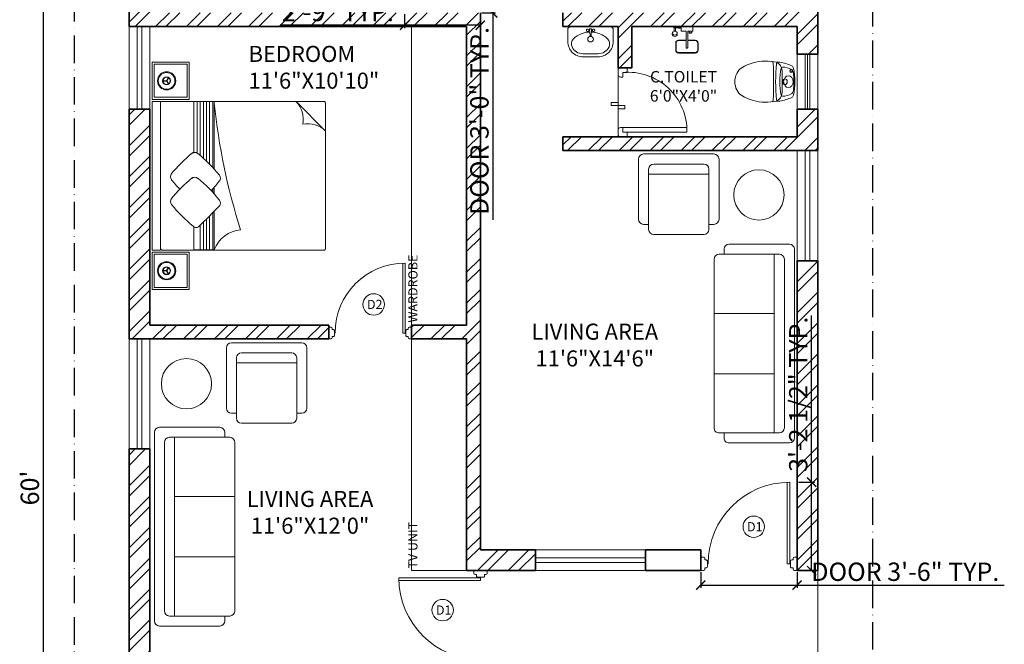
# Model space of a CAD drawing. Units: inches. Extents: x -15 to 1053, y -1 to 793.
# Tile 2 of 8: x 21 to 450, y 337 to 609. Entities that reach past the tile are written whole.
import ezdxf

# ---------------------------------------------------------------- set-up
doc = ezdxf.new("R2010")
doc.units = ezdxf.units.IN
doc.linetypes.add('ACAD_ISO10W100', pattern=[18, 12, -3, 0, -3])
for name, color, linetype, lineweight in [('00 FURNITURE', 15, 'Continuous', 15), ('A-ANNO-DIMS', 2, 'Continuous', 18), ('A-ANNO-TEXT', 7, 'Continuous', 18), ('A-AREA-IDEN', 7, 'Continuous', 18), ('A-DOOR', 4, 'Continuous', 18), ('A-FLOR-CASE', 5, 'Continuous', 18), ('A-FLOR-FIXT', 8, 'Continuous', 13), ('A-FLOR-STRS', 3, 'Continuous', 18), ('A-FURN', 8, 'Continuous', 13), ('A-GLAZ', 4, 'Continuous', 18), ('A-WALL', 7, 'Continuous', 35), ('A-WALL-PATT', 8, 'Continuous', 13), ('A_FUR 1', 5, 'Continuous', 5), ('C-PROP', 1, 'ACAD_ISO10W100', 25)]:
    doc.layers.add(name, color=color, linetype=linetype, lineweight=lineweight)
doc.styles.add('1-100DIM', font='txt', dxfattribs={"height": 0.3})
doc.styles.get("Standard").update_dxf_attribs({"font": 'arial.ttf'})
doc.dimstyles.new('ISO-25', dxfattribs={"dimtxt": 8, "dimasz": 4, "dimexe": 1.25, "dimexo": 0.625, "dimtad": 1, "dimdec": 0, "dimlunit": 4, "dimtxsty": 'Standard', "dimblk": 'ARCHTICK', "dimcen": 3, "dimadec": 0, "dimazin": 0, "dimtfac": 1, "dimtdec": 0, "dimtmove": 0, "dimatfit": 3, "dimldrblk": 'ARCHTICK', "dimfxl": 1, "dimarcsym": 0})

# ---------------------------------------------------------------- blocks, each defined once
blk = doc.blocks.new('s_14')
at = {"extrusion": (0, 0, -1)}
for centre, major_axis, start_param, end_param in [((0, -522), (652, 0), 4.476887, 4.947891), ((0, -522), (652, 0), 4.476887, 4.947891), ((681, -279), (914, 0), 3.289642, 3.481728), ((681, -279), (914, 0), 3.289642, 3.481728), ((-143, -45), (39.1, 0), 3.481728, 4.476887), ((-143, -45), (39.1, 0), 3.481728, 4.476887), ((118, -139), (285, 0), 3.130806, 3.616946), ((-125, -42), (19.2, 0), 3.141593, 9.424778), ((-125, -42), (12.2, 0), 3.141593, 9.424778), ((-97, -51), (42.5, 0), 3.616946, 4.577347), ((0, -624), (766, 0), 4.577347, 4.847431), ((0, -74), (67.1, 0), 3.141593, 9.424778), ((0, -113), (32.9, 0), 3.141593, 9.424778), ((97, -51), (42.5, 0), -1.435755, -0.475353), ((-118, -139), (285, 0), -0.475353, 0.010787), ((143, -45), (39.1, 0), -1.335294, -0.340135), ((143, -45), (39.1, 0), -1.335294, -0.340135), ((-682, -278), (914, 0), -0.340135, -0.148049), ((-682, -278), (914, 0), -0.340135, -0.148049), ((999, -342), (1233, -1), 3.141593, 3.282422), ((999, -342), (1233, -1), 3.141593, 3.282422), ((-87, -187), (137, 0), 3.032389, 3.289642), ((-87, -187), (137, 0), 3.032389, 3.289642), ((-207, -197), (16, 0), 1.680926, 3.032389), ((-207, -197), (16, 0), 1.680926, 3.032389), ((-121, -225), (98.7, 0), 3.365215, 4.657014), ((1, 1302), (1900, -1), 1.460666, 1.680926), ((1, 1302), (1900, -1), 1.460666, 1.680926), ((-149, -142), (17.9, 0), 1.839297, 3.130806), ((0, 291), (579, 0), 1.302296, 1.839297), ((-1, -1970), (2282, -1), 4.657014, 4.767764), ((121, -225), (98.7, 0), -1.515421, -0.223622), ((149, -142), (17.9, 0), 0.010787, 1.302296), ((207, -197), (16, 0), 0.109204, 1.460666), ((207, -197), (16, 0), 0.109204, 1.460666), ((-1000, -341), (1233, -1), -0.140829, 0), ((-1000, -341), (1233, -1), -0.140829, 0), ((87, -187), (137, 0), -0.148049, 0.109204), ((87, -187), (137, 0), -0.148049, 0.109204), ((-210, -263), (19.7, 0), 3.222651, 4.658459), ((-2, -3376), (3914, -2), 4.658459, 4.766319), ((210, -263), (19.7, 0), -1.516867, -0.081058), ((527, -342), (761, 0), 2.693443, 3.141593), ((527, -342), (761, 0), 2.693443, 3.141593), ((-527, -341), (761, 0), 0, 0.44815), ((-527, -341), (761, 0), 0, 0.44815), ((0, -544), (176, 0), 0.44815, 2.693443), ((0, -544), (176, 0), 0.44815, 2.693443)]:
    blk.add_ellipse(centre, major_axis=major_axis, ratio=0.800511, start_param=start_param, end_param=end_param, dxfattribs=at)
blk = doc.blocks.new('s_46')
at = {"ltscale": 600}
h = blk.add_hatch(color=256, dxfattribs=at)
edge = h.paths.add_edge_path()
edge.add_line((13.5, 62), (14.2, 54.1))
edge.add_ellipse((4.2, 52.3), major_axis=(-10.1, 0), ratio=1, start_angle=540, end_angle=550.17546, ccw=False)
edge.add_arc((4.2, 52.3), 10.1, 270, 360, ccw=False)
edge.add_line((4.2, 42.2), (4.2, 41.3))
edge.add_line((4.2, 41.3), (11.9, 41.3))
edge.add_arc((4.2, 52.3), 13.4, 664.69813, 766.48477)
h.paths.add_polyline_path([(4.2, 41.3), (-3.4, 41.3, 0.152567), (4.2, 38.9)])
h.paths.add_polyline_path([(11.9, 41.3), (4.2, 41.3), (4.2, 38.9, 0.152567)])
h.paths.add_polyline_path([(-5.7, 54.1), (-5, 62, 0.475833), (-3.4, 41.3), (4.2, 41.3), (4.2, 42.2, -0.46724)])
for p, q in [((-5.9, 52.3), (-0.7, 110.5)), ((-5.9, 52.3), (-0.7, 110.5)), ((9.1, 110.5), (14.2, 54.1)), ((14.3, 52.3), (9.1, 110.5)), ((14.2, 54.1), (14.3, 52.3))]:
    blk.add_line(p, q, dxfattribs=at)
blk.add_lwpolyline([(-220.8, 171.3, -0.414214), (-70.8, 321.3), (79.2, 321.3, -0.414214), (229.2, 171.3), (229.2, 41.3), (209.2, 21.3), (-200.8, 21.3), (-220.8, 41.3)], format="xyb", close=True, dxfattribs=at)
blk.add_lwpolyline([(12.3, 75.4, 0.181638), (172.2, 141.5, 0.326351), (187.7, 222.7, 0.289814), (79.2, 291.3), (-70.8, 291.3, 0.289814), (-179.2, 222.7, 0.326351), (-163.8, 141.5, 0.181638), (-3.8, 75.4)], format="xyb", dxfattribs=at)
for points in [[(-16.8, 67.4), (-17, 67.5), (-17.2, 67.6), (-17.4, 67.6), (-17.6, 67.7), (-17.8, 67.8), (-18, 67.9), (-18.1, 68.1), (-18.2, 68.2), (-18.3, 68.4), (-18.4, 68.6), (-18.5, 68.8), (-18.7, 68.9), (-18.8, 69.1), (-18.9, 69.2), (-19.1, 69.3), (-19.3, 69.3), (-19.5, 69.3), (-19.7, 69.4), (-19.9, 69.4), (-20.1, 69.4), (-20.3, 69.4), (-20.5, 69.5), (-20.7, 69.6), (-20.8, 69.7), (-21, 69.9), (-21.1, 70), (-21.3, 70.2), (-21.4, 70.3), (-21.5, 70.4), (-21.7, 70.5), (-21.9, 70.5), (-22.1, 70.5), (-22.3, 70.5), (-22.5, 70.5), (-22.7, 70.4), (-22.9, 70.4), (-23.1, 70.4), (-23.3, 70.4), (-23.5, 70.5), (-23.7, 70.6), (-23.9, 70.7), (-24, 70.8), (-24.2, 70.9), (-24.4, 71), (-24.6, 71.1), (-24.7, 71.1), (-24.9, 71.1), (-25.1, 71), (-25.3, 71), (-25.5, 70.9), (-25.7, 70.8), (-25.9, 70.7), (-26.1, 70.6), (-26.3, 70.6), (-26.5, 70.6), (-26.7, 70.6), (-26.9, 70.7), (-27.1, 70.8), (-27.3, 70.8), (-27.5, 70.9), (-27.7, 70.9), (-27.8, 70.9), (-28, 70.8), (-28.2, 70.8), (-28.3, 70.6), (-28.5, 70.5), (-28.7, 70.4), (-28.9, 70.3), (-29.1, 70.2), (-29.3, 70.1), (-29.6, 70.1), (-29.9, 70.1), (-30.2, 70.1), (-30.5, 70), (-30.8, 69.8), (-31.1, 69.5), (-31.4, 69), (-31.6, 68.4), (-32.3, 68.5), (-32.8, 68.4), (-33.2, 68.3), (-33.5, 68.1), (-33.7, 67.8), (-33.9, 67.6), (-34, 67.3), (-34.1, 67.1), (-34.3, 66.9), (-34.5, 66.7), (-34.7, 66.6), (-34.9, 66.5), (-35.1, 66.4), (-35.2, 66.3), (-35.4, 66.2), (-35.5, 66), (-35.6, 65.9), (-35.6, 65.7), (-35.7, 65.5), (-35.7, 65.3), (-35.7, 65.1), (-35.8, 64.9), (-35.8, 64.7), (-35.9, 64.5), (-36, 64.3), (-36.2, 64.2), (-36.3, 64), (-36.5, 63.9), (-36.6, 63.8), (-36.8, 63.6), (-36.9, 63.5), (-37, 63.3), (-37, 63.1), (-37, 63), (-37, 62.8), (-37, 62.6), (-37, 62.3), (-37, 62.1), (-37, 61.9), (-37, 61.7), (-37.1, 61.5), (-37.2, 61.4), (-37.3, 61.2), (-37.4, 61), (-37.5, 60.8), (-37.6, 60.7), (-37.7, 60.5), (-37.8, 60.3), (-37.8, 60.1), (-37.7, 60), (-37.7, 59.8), (-37.6, 59.6), (-37.5, 59.4), (-37.4, 59.2), (-37.4, 59), (-37.4, 58.8), (-37.4, 58.6), (-37.4, 58.4), (-37.5, 58.2), (-37.6, 58), (-37.7, 57.8), (-37.7, 57.6), (-37.8, 57.4), (-37.8, 57.2), (-37.7, 57.1), (-37.6, 56.9), (-37.5, 56.7), (-37.4, 56.6), (-37.3, 56.4), (-37.2, 56.2), (-37.1, 56), (-37, 55.8), (-37, 55.6), (-37, 55.4), (-37, 55.2), (-37, 55), (-37, 54.8), (-37, 54.6), (-37, 54.4), (-37, 54.2), (-36.9, 54.1), (-36.8, 53.9), (-36.6, 53.8), (-36.5, 53.7), (-36.3, 53.5), (-36.2, 53.4), (-36, 53.2), (-35.9, 53.1), (-35.8, 52.9), (-35.8, 52.7), (-35.7, 52.5), (-35.7, 52.3), (-35.7, 52.1), (-35.6, 51.9), (-35.6, 51.7), (-35.5, 51.5), (-35.4, 51.4), (-35.2, 51.3), (-35.1, 51.2), (-34.9, 51.1), (-34.7, 51), (-34.5, 50.9), (-34.3, 50.8), (-34.2, 50.7), (-34, 50.5), (-33.9, 50.3), (-33.8, 50.1), (-33.8, 49.9), (-33.7, 49.8), (-33.6, 49.6), (-33.5, 49.4), (-33.4, 49.3), (-33.2, 49.2), (-33.1, 49.1), (-32.9, 49.1), (-32.7, 49), (-32.5, 49), (-32.2, 48.9), (-32.1, 48.9), (-31.9, 48.8), (-31.7, 48.7), (-31.6, 48.5), (-31.4, 48.3), (-31.3, 48.2), (-31.2, 48), (-31.1, 47.9), (-30.9, 47.7), (-30.8, 47.6), (-30.6, 47.6), (-30.4, 47.5), (-30.2, 47.5), (-30, 47.6), (-29.8, 47.6), (-29.6, 47.6), (-29.4, 47.6), (-29.2, 47.5), (-29, 47.4), (-28.8, 47.3), (-28.7, 47.2), (-28.5, 47.1), (-28.3, 46.9), (-28.2, 46.8), (-28, 46.7), (-27.8, 46.7), (-27.7, 46.7), (-27.5, 46.7), (-27.3, 46.7), (-27.1, 46.8), (-26.9, 46.9), (-26.7, 46.9), (-26.5, 47), (-26.3, 47), (-26.1, 46.9), (-25.9, 46.9), (-25.7, 46.8), (-25.5, 46.7), (-25.3, 46.6), (-25.1, 46.5), (-24.9, 46.5), (-24.7, 46.5), (-24.6, 46.5), (-24.4, 46.6), (-24.2, 46.7), (-24, 46.8), (-23.9, 46.9), (-23.7, 47), (-23.5, 47.1), (-23.3, 47.1), (-23.1, 47.2), (-22.9, 47.2), (-22.7, 47.1), (-22.5, 47.1), (-22.3, 47), (-22.1, 47), (-21.9, 47), (-21.7, 47.1), (-21.5, 47.1), (-21.4, 47.2), (-21.3, 47.4), (-21.1, 47.5), (-21, 47.7), (-20.8, 47.8), (-20.7, 48), (-20.5, 48.1), (-20.3, 48.1), (-20.1, 48.2), (-19.9, 48.2), (-19.7, 48.2), (-19.5, 48.2), (-19.3, 48.2), (-19.1, 48.3), (-18.9, 48.4), (-18.8, 48.5), (-18.7, 48.6), (-18.5, 48.8), (-18.4, 49), (-18.3, 49.2), (-18.2, 49.3), (-18.1, 49.5), (-18, 49.7), (-17.8, 49.8), (-17.6, 49.9), (-17.4, 49.9), (-17.2, 50), (-17, 50.1), (-16.8, 50.1), (-16.7, 50.2), (-16.5, 50.3), (-16.4, 50.5), (-16.3, 50.7), (-16.3, 50.8), (-16.2, 51), (-16.2, 51.3), (-16.1, 51.5), (-16, 51.6), (-15.9, 51.8), (-15.8, 52), (-15.6, 52.1), (-15.5, 52.2), (-15.3, 52.3), (-15.1, 52.4), (-15, 52.6), (-14.8, 52.7), (-14.7, 52.8), (-14.7, 53), (-14.6, 53.2), (-14.6, 53.4), (-14.6, 53.6), (-14.6, 53.8), (-14.6, 54), (-14.6, 54.2), (-14.5, 54.4), (-14.4, 54.6), (-14.3, 54.8), (-14.2, 54.9), (-14, 55.1), (-13.9, 55.2), (-13.7, 55.4), (-13.6, 55.5), (-13.6, 55.7), (-13.6, 55.9), (-13.6, 56.1), (-13.6, 56.3), (-13.7, 56.5), (-13.7, 56.7), (-13.8, 56.9), (-13.8, 57.1), (-13.8, 57.3), (-13.7, 57.5), (-13.7, 57.7), (-13.6, 57.9), (-13.5, 58.1), (-13.4, 58.2), (-13.3, 58.4), (-13.2, 58.6), (-13.2, 58.8), (-13.2, 59), (-13.3, 59.1), (-13.4, 59.3), (-13.5, 59.5), (-13.6, 59.7), (-13.7, 59.9), (-13.7, 60.1), (-13.8, 60.3), (-13.8, 60.5), (-13.8, 60.7), (-13.7, 60.9), (-13.7, 61.1), (-13.6, 61.3), (-13.6, 61.5), (-13.6, 61.7), (-13.6, 61.9), (-13.6, 62), (-13.7, 62.2), (-13.9, 62.3), (-14, 62.5), (-14.2, 62.6), (-14.3, 62.8), (-14.4, 63), (-14.5, 63.1), (-14.6, 63.3), (-14.6, 63.5), (-14.6, 63.8), (-14.6, 64), (-14.6, 64.2), (-14.6, 64.4), (-14.7, 64.6), (-14.7, 64.7), (-14.8, 64.9), (-15, 65), (-15.1, 65.1), (-15.3, 65.2), (-15.5, 65.3), (-15.6, 65.5), (-15.8, 65.6), (-15.9, 65.7), (-16, 65.9), (-16.1, 66.1), (-16.2, 66.3), (-16.2, 66.5), (-16.3, 66.7), (-16.3, 66.9), (-16.4, 67.1), (-16.5, 67.2), (-16.7, 67.3)], [(22.1, 61.1), (22, 61.3), (22, 61.5), (22, 61.7), (22, 61.9), (22.1, 62), (22.2, 62.2), (22.3, 62.3), (22.4, 62.5), (22.6, 62.6), (22.7, 62.8), (22.8, 63), (22.9, 63.1), (23, 63.3), (23, 63.5), (23, 63.8), (23, 64), (23, 64.2), (23, 64.4), (23.1, 64.6), (23.1, 64.7), (23.2, 64.9), (23.4, 65), (23.5, 65.1), (23.7, 65.2), (23.9, 65.3), (24.1, 65.5), (24.2, 65.6), (24.4, 65.7), (24.5, 65.9), (24.5, 66.1), (24.6, 66.3), (24.7, 66.5), (24.7, 66.7), (24.8, 66.9), (24.9, 67.1), (25, 67.2), (25.1, 67.3), (25.3, 67.4), (25.4, 67.5), (25.6, 67.6), (25.8, 67.6), (26, 67.7), (26.2, 67.8), (26.4, 67.9), (26.5, 68.1), (26.7, 68.2), (26.8, 68.4), (26.9, 68.6), (27, 68.8), (27.1, 68.9), (27.2, 69.1), (27.3, 69.2), (27.5, 69.3), (27.7, 69.3), (27.9, 69.3), (28.1, 69.4), (28.3, 69.4), (28.5, 69.4), (28.7, 69.4), (28.9, 69.5), (29.1, 69.6), (29.2, 69.7), (29.4, 69.9), (29.5, 70), (29.7, 70.2), (29.8, 70.3), (30, 70.4), (30.1, 70.5), (30.3, 70.5), (30.5, 70.5), (30.7, 70.5), (30.9, 70.5), (31.1, 70.4), (31.3, 70.4), (31.5, 70.4), (31.7, 70.4), (31.9, 70.5), (32.1, 70.6), (32.3, 70.7), (32.5, 70.8), (32.6, 70.9), (32.8, 71), (33, 71.1), (33.2, 71.1), (33.4, 71.1), (33.5, 71), (33.7, 71), (33.9, 70.9), (34.1, 70.8), (34.3, 70.7), (34.5, 70.6), (34.7, 70.6), (34.9, 70.6), (35.1, 70.6), (35.3, 70.7), (35.5, 70.8), (35.7, 70.8), (35.9, 70.9), (36.1, 70.9), (36.3, 70.9), (36.4, 70.8), (36.6, 70.8), (36.8, 70.6), (36.9, 70.5), (37.1, 70.4), (37.3, 70.3), (37.5, 70.2), (37.8, 70.1), (38, 70.1), (38.3, 70.1), (38.6, 70.1), (38.9, 70), (39.2, 69.8), (39.5, 69.5), (39.8, 69), (40.1, 68.4), (40.7, 68.5), (41.3, 68.4), (41.7, 68.3), (42, 68.1), (42.2, 67.8), (42.3, 67.6), (42.4, 67.3), (42.6, 67.1), (42.7, 66.9), (42.9, 66.7), (43.1, 66.6), (43.3, 66.5), (43.5, 66.4), (43.6, 66.3), (43.8, 66.2), (43.9, 66), (44, 65.9), (44.1, 65.7), (44.1, 65.5), (44.1, 65.3), (44.2, 65.1), (44.2, 64.9), (44.2, 64.7), (44.3, 64.5), (44.4, 64.3), (44.6, 64.2), (44.7, 64), (44.9, 63.9), (45.1, 63.8), (45.2, 63.6), (45.3, 63.5), (45.4, 63.3), (45.5, 63.1), (45.5, 63), (45.5, 62.8), (45.4, 62.6), (45.4, 62.3), (45.4, 62.1), (45.4, 61.9), (45.4, 61.7), (45.5, 61.5), (45.6, 61.4), (45.7, 61.2), (45.8, 61), (46, 60.8), (46.1, 60.7), (46.1, 60.5), (46.2, 60.3), (46.2, 60.1), (46.1, 60), (46.1, 59.8), (46, 59.6), (45.9, 59.4), (45.9, 59.2), (45.8, 59), (45.8, 58.8), (45.8, 58.6), (45.9, 58.4), (45.9, 58.2), (46, 58), (46.1, 57.8), (46.1, 57.6), (46.2, 57.4), (46.2, 57.2), (46.1, 57.1), (46.1, 56.9), (46, 56.7), (45.8, 56.6), (45.7, 56.4), (45.6, 56.2), (45.5, 56), (45.4, 55.8), (45.4, 55.6), (45.4, 55.4), (45.4, 55.2), (45.4, 55), (45.5, 54.8), (45.5, 54.6), (45.5, 54.4), (45.4, 54.2), (45.3, 54.1), (45.2, 53.9), (45.1, 53.8), (44.9, 53.7), (44.7, 53.5), (44.6, 53.4), (44.4, 53.2), (44.3, 53.1), (44.2, 52.9), (44.2, 52.7), (44.2, 52.5), (44.1, 52.3), (44.1, 52.1), (44.1, 51.9), (44, 51.7), (43.9, 51.5), (43.8, 51.4), (43.6, 51.3), (43.5, 51.2), (43.3, 51.1), (43.1, 51), (42.9, 50.9), (42.7, 50.8), (42.6, 50.7), (42.5, 50.5), (42.4, 50.3), (42.3, 50.1), (42.2, 49.9), (42.1, 49.8), (42, 49.6), (41.9, 49.4), (41.8, 49.3), (41.7, 49.2), (41.5, 49.1), (41.3, 49.1), (41.1, 49), (40.9, 49), (40.7, 48.9), (40.5, 48.9), (40.3, 48.8), (40.1, 48.7), (40, 48.5), (39.9, 48.3), (39.7, 48.2), (39.6, 48), (39.5, 47.9), (39.4, 47.7), (39.2, 47.6), (39, 47.6), (38.8, 47.5), (38.6, 47.5), (38.4, 47.6), (38.2, 47.6), (38, 47.6), (37.8, 47.6), (37.6, 47.5), (37.4, 47.4), (37.2, 47.3), (37.1, 47.2), (36.9, 47.1), (36.8, 46.9), (36.6, 46.8), (36.4, 46.7), (36.3, 46.7), (36.1, 46.7), (35.9, 46.7), (35.7, 46.7), (35.5, 46.8), (35.3, 46.9), (35.1, 46.9), (34.9, 47), (34.7, 47), (34.5, 46.9), (34.3, 46.9), (34.1, 46.8), (33.9, 46.7), (33.7, 46.6), (33.5, 46.5), (33.4, 46.5), (33.2, 46.5), (33, 46.5), (32.8, 46.6), (32.6, 46.7), (32.5, 46.8), (32.3, 46.9), (32.1, 47), (31.9, 47.1), (31.7, 47.1), (31.5, 47.2), (31.3, 47.2), (31.1, 47.1), (30.9, 47.1), (30.7, 47), (30.5, 47), (30.3, 47), (30.1, 47.1), (30, 47.1), (29.8, 47.2), (29.7, 47.4), (29.5, 47.5), (29.4, 47.7), (29.2, 47.8), (29.1, 48), (28.9, 48.1), (28.7, 48.1), (28.5, 48.2), (28.3, 48.2), (28.1, 48.2), (27.9, 48.2), (27.7, 48.2), (27.5, 48.3), (27.3, 48.4), (27.2, 48.5), (27.1, 48.6), (27, 48.8), (26.9, 49), (26.8, 49.2), (26.7, 49.3), (26.5, 49.5), (26.4, 49.7), (26.2, 49.8), (26, 49.9), (25.8, 49.9), (25.6, 50), (25.4, 50.1), (25.3, 50.1), (25.1, 50.2), (25, 50.3), (24.9, 50.5), (24.8, 50.7), (24.7, 50.8), (24.7, 51), (24.6, 51.3), (24.5, 51.5), (24.5, 51.6), (24.4, 51.8), (24.2, 52), (24.1, 52.1), (23.9, 52.2), (23.7, 52.3), (23.5, 52.4), (23.4, 52.6), (23.2, 52.7), (23.1, 52.8), (23.1, 53), (23, 53.2), (23, 53.4), (23, 53.6), (23, 53.8), (23, 54), (23, 54.2), (22.9, 54.4), (22.8, 54.6), (22.7, 54.8), (22.6, 54.9), (22.4, 55.1), (22.3, 55.2), (22.2, 55.4), (22.1, 55.5), (22, 55.7), (22, 55.9), (22, 56.1), (22, 56.3), (22.1, 56.5), (22.1, 56.7), (22.2, 56.9), (22.2, 57.1), (22.2, 57.3), (22.2, 57.5), (22.1, 57.7), (22, 57.9), (21.9, 58.1), (21.8, 58.2), (21.7, 58.4), (21.6, 58.6), (21.6, 58.8), (21.6, 59), (21.7, 59.1), (21.8, 59.3), (21.9, 59.5), (22, 59.7), (22.1, 59.9), (22.2, 60.1), (22.2, 60.3), (22.2, 60.5), (22.2, 60.7), (22.1, 60.9)]]:
    blk.add_lwpolyline(points, close=True, dxfattribs=at)
blk.add_circle((4.2, 146.3), 28, dxfattribs=at)
for centre, radius, start, end in [((4.2, 108.2), 5.42, 24.6783, 155.3217), ((4.2, 52.3), 10.1, 169.82454, 0)]:
    blk.add_arc(centre, radius, start, end, dxfattribs=at)
for centre, major_axis, ratio, start_param, end_param in [((4.2, 110.5), (-4.93, 0), 0.641024, 3.141593, 6.283185), ((4.2, 52.3), (-10.1, 0), 1, 6.10559, 9.602373)]:
    blk.add_ellipse(centre, major_axis=major_axis, ratio=ratio, start_param=start_param, end_param=end_param, dxfattribs=at)
blk = doc.blocks.new('A$C7A0926BE')
for p, q in [((-6.55, 0), (-5.57, 0)), ((-6.55, -0.65), (-6.55, 0)), ((-5.57, 0), (-5.57, -0.65)), ((-2.89, 0), (-2.89, -2.29)), ((2.89, 0), (-2.89, 0)), ((2.89, -2.29), (2.89, 0)), ((-7.32, -3.29), (-7.32, -3.94)), ((-5.57, -0.65), (-6.55, -0.65)), ((-6.34, -0.65), (-5.74, -0.65)), ((-6.34, -2.33), (-6.34, -0.65)), ((-5.74, -2.33), (-6.34, -2.33)), ((-5.74, -0.65), (-5.74, -2.33)), ((-5.57, -0.28), (-2.89, -0.56)), ((-5.57, -0.65), (-2.89, -0.94)), ((-4.84, -3.94), (-4.85, -3.29)), ((-2.89, -2.29), (-0.45, -2.29)), ((0.39, -2.29), (2.89, -2.29)), ((1.04, -2.29), (1.04, -3.12)), ((2.37, -2.29), (1.04, -2.29)), ((1.04, -3.12), (2.37, -3.12)), ((1.13, -3.12), (1.13, -3.23)), ((2.3, -3.12), (1.13, -3.12)), ((1.13, -3.23), (2.3, -3.23)), ((2.3, -3.23), (2.3, -3.12)), ((2.37, -3.12), (2.37, -2.29))]:
    blk.add_line(p, q)
at = {"ltscale": 100}
for p, q in [((-0.45, -10.48), (-0.45, -2.29)), ((0.39, -10.48), (0.39, -2.29)), ((0.18, -10.69), (-0.24, -10.69))]:
    blk.add_line(p, q, dxfattribs=at)
for points in [[(-0.45, -6.79), (-4.23, -6.79, 0.414214), (-5.63, -8.19), (-5.63, -11.8, 0.414214), (-4.23, -13.2), (4.17, -13.2, 0.414214), (5.57, -11.8), (5.57, -8.19, 0.414214), (4.17, -6.79), (0.39, -6.79)], [(-0.45, -7), (-4.23, -7, 0.414214), (-5.42, -8.19), (-5.42, -11.8, 0.414214), (-4.23, -12.99), (4.17, -12.99, 0.414214), (5.36, -11.8), (5.36, -8.19, 0.414214), (4.17, -7), (0.39, -7)]]:
    blk.add_lwpolyline(points, format="xyb", dxfattribs=at)
for centre, start, end in [((-0.24, -10.48), 180, 270), ((0.18, -10.48), 270, 0)]:
    blk.add_arc(centre, 0.21, start, end, dxfattribs=at)
at = {"extrusion": (0, 0, -1)}
blk.add_ellipse((-6.08, -3.29), major_axis=(-1.24, 0), ratio=0.790849, dxfattribs=at)
blk.add_ellipse((-6.08, -3.94), major_axis=(-1.24, 0), ratio=0.790849, start_param=3.141593, end_param=6.283185, dxfattribs=at)
blk = doc.blocks.new('ESTSET')
at = {"layer": 'A_FUR 1'}
for p, q in [((-10.44, 4.1), (-10.44, 32.1)), ((-8.44, 4.1), (-8.44, 32.1)), ((-36.44, 6.1), (-36.44, 3.1)), ((-34.44, 6.1), (-36.44, 6.1)), ((-34.44, 4.1), (-34.44, 6.1)), ((-34.44, 4.1), (-34.44, 6.1)), ((-8.44, 4.1), (-8.44, 6.1)), ((-8.44, 6.1), (-6.44, 6.1)), ((-8.44, 4.1), (-8.44, 6.1)), ((-6.44, 6.1), (-6.44, 3.1)), ((-6.44, 2.1), (-36.44, 2.1)), ((-35.44, 2.1), (-33.44, 2.1)), ((-32.44, 4.1), (-34.44, 4.1)), ((-32.44, 4.1), (-34.44, 4.1)), ((-32.44, 3.1), (-32.44, 4.1)), ((-10.44, 3.1), (-10.44, 4.1)), ((-10.44, 4.1), (-8.44, 4.1)), ((-10.44, 4.1), (-8.44, 4.1)), ((-7.44, 2.1), (-9.44, 2.1))]:
    blk.add_line(p, q, dxfattribs=at)
for points in [[(-21.44, 2.1), (-18.67, 2.1), (-18.67, 5.1), (-20.06, 5.1)], [(-20.06, 5.1), (-20.06, -0.91)], [(-21.44, 2.1), (-21.44, -0.91), (-20.06, -0.91)]]:
    blk.add_lwpolyline(points, dxfattribs=at)
for centre, radius, start, end in [((-8.91, 6.46), 25.64, 88.9606, 185.2816), ((-35.44, 3.1), 1, 180, 270), ((-33.44, 3.1), 1, 270, 0), ((-9.44, 3.1), 1, 180, 270), ((-7.44, 3.1), 1, 270, 0)]:
    blk.add_arc(centre, radius, start, end, dxfattribs=at)
blk = doc.blocks.new('DDD')
at = {"layer": '00 FURNITURE'}
for p, q in [((-12579.77, -15859.53), (-12579.77, -15829.05)), ((-12578.77, -15859.53), (-12578.77, -15829.03)), ((-12612.02, -15857.03), (-12612.02, -15862.03)), ((-12611.02, -15857.03), (-12612.02, -15857.03)), ((-12610.52, -15858.03), (-12610.52, -15857.53)), ((-12578.77, -15859.53), (-12579.77, -15859.53)), ((-12577.52, -15858.03), (-12577.52, -15857.53)), ((-12577.02, -15857.03), (-12576.02, -15857.03)), ((-12576.02, -15857.03), (-12576.02, -15862.03)), ((-12612.02, -15862.03), (-12611.02, -15862.03)), ((-12610.52, -15861.53), (-12610.52, -15861.03)), ((-12577.52, -15861.53), (-12577.52, -15861.03)), ((-12576.02, -15862.03), (-12577.02, -15862.03))]:
    blk.add_line(p, q, dxfattribs=at)
for points in [[(-12610.52, -15861.03), (-12610.02, -15861.03, 0.414214), (-12609.52, -15860.53), (-12609.52, -15858.53, 0.414214), (-12610.02, -15858.03), (-12610.52, -15858.03)], [(-12577.52, -15861.03), (-12578.02, -15861.03, -0.414214), (-12578.52, -15860.53), (-12578.52, -15858.53, -0.414214), (-12578.02, -15858.03), (-12577.52, -15858.03)]]:
    blk.add_lwpolyline(points, format="xyb", dxfattribs=at)
for centre, radius, start, end in [((-12578.77, -15859.53), 30.5, 90, 180), ((-12611.02, -15857.53), 0.5, 0, 90), ((-12577.02, -15857.53), 0.5, 90, 180), ((-12611.02, -15861.53), 0.5, 270, 0), ((-12577.02, -15861.53), 0.5, 180, 270)]:
    blk.add_arc(centre, radius, start, end, dxfattribs=at)
blk = doc.blocks.new('RGWTG')
at = {"layer": '00 FURNITURE'}
for p, q in [((578.23, 3473.51), (577.36, 3475.01)), ((578.36, 3473.58), (577.49, 3475.09)), ((578.23, 3473.58), (577.36, 3472.08)), ((578.36, 3473.51), (577.49, 3472)), ((578.29, 3473.62), (580.03, 3473.62)), ((578.29, 3473.47), (580.03, 3473.47)), ((521.93, 3464.58), (509.03, 3451.68)), ((509.03, 3422.63), (509.03, 3463.68)), ((509.93, 3464.58), (566.4, 3464.58)), ((557.53, 3463.84), (557.53, 3464.49)), ((557.53, 3464.49), (566.4, 3464.49)), ((558.2, 3464.49), (558.2, 3435.82)), ((559.57, 3464.49), (559.57, 3437.25)), ((560.94, 3464.49), (560.94, 3438.58)), ((562.3, 3464.49), (562.3, 3439.83)), ((563.67, 3464.49), (563.67, 3440.99)), ((565.04, 3464.49), (565.04, 3442.08)), ((566.4, 3464.58), (580.98, 3464.58)), ((566.4, 3464.49), (566.4, 3442.08)), ((566.4, 3464.49), (566.4, 3463.84)), ((580.98, 3464.58), (580.98, 3416.72)), ((558.2, 3426.48), (558.2, 3425.04)), ((509.03, 3400.68), (509.03, 3422.63)), ((558.2, 3416.13), (558.2, 3399.95)), ((559.57, 3414.75), (559.57, 3399.95)), ((580.98, 3416.72), (580.98, 3400.68)), ((560.94, 3413.39), (560.94, 3399.95)), ((562.3, 3412.04), (562.3, 3399.95)), ((563.67, 3410.72), (563.67, 3399.95)), ((580.08, 3399.78), (509.93, 3399.78)), ((557.53, 3399.95), (557.53, 3400.6)), ((566.4, 3399.95), (557.53, 3399.95)), ((566.4, 3400.6), (566.4, 3399.95)), ((578.23, 3390.78), (577.36, 3392.29)), ((578.23, 3390.86), (577.36, 3389.36)), ((578.36, 3390.86), (577.49, 3392.36)), ((578.36, 3390.78), (577.49, 3389.28)), ((578.29, 3390.9), (580.03, 3390.9)), ((578.29, 3390.74), (580.03, 3390.74))]:
    blk.add_line(p, q, dxfattribs=at)
for points in [[(568.43, 3465.48), (584.63, 3465.48), (584.63, 3481.68), (568.43, 3481.68)], [(569.33, 3466.38), (583.73, 3466.38), (583.73, 3480.78), (569.33, 3480.78)], [(580.98, 3399.78), (584.63, 3399.78), (584.63, 3464.58), (580.98, 3464.58)], [(568.43, 3398.88), (584.63, 3398.88), (584.63, 3382.68), (568.43, 3382.68)], [(569.33, 3397.98), (583.73, 3397.98), (583.73, 3383.58), (569.33, 3383.58)]]:
    blk.add_lwpolyline(points, close=True, dxfattribs=at)
for points in [[(566.52, 3464.49), (557.53, 3464.49), (557.53, 3435.08)], [(557.53, 3427.21), (557.53, 3424.3)], [(557.53, 3416.82), (557.53, 3399.95), (566.4, 3399.95), (566.4, 3409.94)]]:
    blk.add_lwpolyline(points, dxfattribs=at)
for centre, radius in [((578.29, 3473.54), 3.97), ((578.29, 3473.54), 3.63), ((578.29, 3473.54), 1.74), ((578.29, 3473.54), 1.56), ((578.29, 3390.82), 3.97), ((578.29, 3390.82), 3.63), ((578.29, 3390.82), 1.74), ((578.29, 3390.82), 1.56)]:
    blk.add_circle(centre, radius, dxfattribs=at)
for centre, radius, start, end in [((509.93, 3463.68), 0.9, 90, 180), ((529.65, 3456.88), 10.9, 135.0361, 191.9278), ((290.56, 3490.52), 268.3, 342.2214, 354.2925), ((516.73, 3443.97), 10.9, 78.0722, 134.9639), ((598.15, 3399.01), 54.32, 127.931, 142.069), ((566.05, 3440.57), 1.82, 45, 135), ((533.58, 3399.31), 54.32, 37.931, 52.069), ((556.59, 3431.11), 1.82, 135, 225), ((566.05, 3429.78), 1.82, 45, 135), ((533.58, 3388.53), 54.32, 37.931, 52.069), ((574.84, 3431.77), 1.82, 315, 45), ((597.87, 3463.6), 54.32, 217.931, 224.141), ((598.15, 3388.23), 54.32, 127.931, 142.069), ((533.28, 3463.88), 54.32, 316.32, 322.069), ((556.59, 3420.33), 1.82, 135, 225), ((765.33, 3619.75), 290.45, 223.6069, 226.2326), ((533.28, 3453.1), 54.32, 307.931, 322.069), ((574.84, 3420.99), 1.82, 315, 45), ((565.44, 3411.05), 1.47, 225.9674, 326.8337), ((545.02, 3395.29), 13.35, 20.4224, 85.5825), ((509.93, 3400.68), 0.9, 180, 270), ((580.08, 3400.68), 0.9, 270, 0)]:
    blk.add_arc(centre, radius, start, end, dxfattribs=at)
blk = doc.blocks.new('sofa 6')
for p, q in [((-1044, 890), (1044, 890)), ((-1100, 167), (-1100, 834)), ((-933, 779), (933, 779)), ((1100, 834), (1100, 167)), ((-989, 56), (-989, 723)), ((-989, 667), (989, 667)), ((-334, 667), (-334, 0)), ((334, 667), (334, 0)), ((989, 723), (989, 56)), ((-989, 111), (-1044, 111)), ((1044, 111), (989, 111)), ((933, 0), (-933, 0))]:
    blk.add_line(p, q)
for centre, start, end in [((-1044, 834), 90, 180), ((1044, 834), 0, 90), ((-933, 723), 90, 180), ((933, 723), 0, 90), ((-1044, 167), 180, 270), ((1044, 167), 270, 0), ((-933, 56), 180, 270), ((933, 56), 270, 0)]:
    blk.add_arc(centre, 55.6, start, end)
blk = doc.blocks.new('_ArchTick')
at = {"color": 0, "linetype": 'ByBlock', "const_width": 0.15}
blk.add_lwpolyline([(-0.5, -0.5), (0.5, 0.5)], dxfattribs=at)
blk = doc.blocks.new('*D17')
at = {"layer": 'A-ANNO-DIMS', "color": 0, "lineweight": -2, "transparency": 16777216}
for p, q in [((44.24, 764.76), (30.11, 764.76)), ((31.36, 764.76), (31.36, 44.76)), ((44.24, 44.76), (30.11, 44.76))]:
    blk.add_line(p, q, dxfattribs=at)
at = {"layer": 'Defpoints', "color": 0, "transparency": 16777216}
for p in [(44.87, 764.76), (31.36, 44.76), (44.87, 44.76)]:
    blk.add_point(p, dxfattribs=at)
at = {"layer": 'A-ANNO-DIMS', "color": 0, "lineweight": -2, "transparency": 16777216, "xscale": 4, "yscale": 4, "zscale": 4}
for p, rotation in [((31.36, 764.76), 90), ((31.36, 44.76), 270)]:
    blk.add_blockref('_ArchTick', p, dxfattribs=dict(at, rotation=rotation))
at = {"layer": 'A-ANNO-DIMS', "color": 0, "transparency": 16777216, "insert": (26.65, 404.76), "char_height": 8, "attachment_point": 5, "rotation": 90}
blk.add_mtext("60'", dxfattribs=at)
blk = doc.blocks.new('ARMCHAIR')
for p, q in [((2.19, 30.66), (32.85, 30.66)), ((0, 2.19), (0, 28.47)), ((6.57, 26.28), (28.47, 26.28)), ((35.04, 28.47), (35.04, 2.19)), ((4.38, -2.19), (4.38, 24.09)), ((30.66, 24.09), (30.66, -2.19)), ((4.38, 0), (2.19, 0)), ((32.85, 0), (30.66, 0)), ((28.47, -4.38), (6.57, -4.38))]:
    blk.add_line(p, q)
for centre, start, end in [((2.19, 28.47), 90, 180), ((32.85, 28.47), 0, 90), ((6.57, 24.09), 90, 180), ((28.47, 24.09), 0, 90), ((2.19, 2.19), 180, 270), ((32.85, 2.19), 270, 0), ((6.57, -2.19), 180, 270), ((28.47, -2.19), 270, 0)]:
    blk.add_arc(centre, 2.19, start, end)
blk = doc.blocks.new('*D32')
at = {"layer": 'A-ANNO-DIMS', "color": 0, "lineweight": -2, "transparency": 16777216}
for p, q in [((317.87, 368.14), (317.87, 361.21)), ((359.87, 368.14), (359.87, 361.21)), ((317.87, 362.46), (359.87, 362.46)), ((359.87, 362.46), (450.12, 362.46))]:
    blk.add_line(p, q, dxfattribs=at)
at = {"layer": 'Defpoints', "color": 0, "transparency": 16777216}
for p in [(317.87, 368.76), (359.87, 368.76), (359.87, 362.46)]:
    blk.add_point(p, dxfattribs=at)
at = {"layer": 'A-ANNO-DIMS', "color": 0, "lineweight": -2, "transparency": 16777216, "xscale": 4, "yscale": 4, "zscale": 4, "rotation": 180}
blk.add_blockref('_ArchTick', (317.87, 362.46), dxfattribs=at)
at = {"layer": 'A-ANNO-DIMS', "color": 0, "lineweight": -2, "transparency": 16777216, "xscale": 4, "yscale": 4, "zscale": 4}
blk.add_blockref('_ArchTick', (359.87, 362.46), dxfattribs=at)
at = {"layer": 'A-ANNO-DIMS', "color": 0, "transparency": 16777216, "insert": (406.99, 367.23), "char_height": 8, "attachment_point": 5}
blk.add_mtext('DOOR 3\'-6" TYP.', dxfattribs=at)
blk = doc.blocks.new('*D33')
at = {"layer": 'A-ANNO-DIMS', "color": 0, "lineweight": -2, "transparency": 16777216}
for p, q in [((366.17, 407.26), (366.17, 479.91)), ((360.49, 407.26), (367.42, 407.26)), ((366.17, 368.76), (366.17, 407.26)), ((360.49, 368.76), (367.42, 368.76))]:
    blk.add_line(p, q, dxfattribs=at)
at = {"layer": 'Defpoints', "color": 0, "transparency": 16777216}
for p in [(359.87, 407.26), (366.17, 407.26), (359.87, 368.76)]:
    blk.add_point(p, dxfattribs=at)
at = {"layer": 'A-ANNO-DIMS', "color": 0, "lineweight": -2, "transparency": 16777216, "xscale": 4, "yscale": 4, "zscale": 4}
for p, rotation in [((366.17, 407.26), 90), ((366.17, 368.76), 270)]:
    blk.add_blockref('_ArchTick', p, dxfattribs=dict(at, rotation=rotation))
at = {"layer": 'A-ANNO-DIMS', "color": 0, "transparency": 16777216, "insert": (361.4, 445.59), "char_height": 8, "attachment_point": 5, "rotation": 90}
blk.add_mtext('3\'-2 1/2" TYP.', dxfattribs=at)
blk = doc.blocks.new('*D34')
at = {"layer": 'A-ANNO-DIMS', "color": 0, "lineweight": -2, "transparency": 16777216}
for p, q in [((222.49, 647.76), (228.52, 647.76)), ((227.27, 647.76), (227.27, 611.76)), ((222.49, 611.76), (228.52, 611.76)), ((227.27, 611.76), (227.27, 521.52))]:
    blk.add_line(p, q, dxfattribs=at)
at = {"layer": 'Defpoints', "color": 0, "transparency": 16777216}
for p in [(221.87, 647.76), (221.87, 611.76), (227.27, 611.76)]:
    blk.add_point(p, dxfattribs=at)
at = {"layer": 'A-ANNO-DIMS', "color": 0, "lineweight": -2, "transparency": 16777216, "xscale": 4, "yscale": 4, "zscale": 4}
for p, rotation in [((227.27, 647.76), 90), ((227.27, 611.76), 270)]:
    blk.add_blockref('_ArchTick', p, dxfattribs=dict(at, rotation=rotation))
at = {"layer": 'A-ANNO-DIMS', "color": 0, "transparency": 16777216, "insert": (222.5, 564.64), "char_height": 8, "attachment_point": 5, "rotation": 90}
blk.add_mtext('DOOR 3\'-0" TYP.', dxfattribs=at)
blk = doc.blocks.new('*D35')
at = {"layer": 'A-ANNO-DIMS', "color": 0, "lineweight": -2, "transparency": 16777216}
for p, q in [((188.87, 611.14), (188.87, 605.11)), ((221.87, 611.14), (221.87, 605.11)), ((188.87, 606.36), (134.72, 606.36)), ((221.87, 606.36), (188.87, 606.36))]:
    blk.add_line(p, q, dxfattribs=at)
at = {"layer": 'Defpoints', "color": 0, "transparency": 16777216}
for p in [(188.87, 611.76), (221.87, 611.76), (188.87, 606.36)]:
    blk.add_point(p, dxfattribs=at)
at = {"layer": 'A-ANNO-DIMS', "color": 0, "lineweight": -2, "transparency": 16777216, "xscale": 4, "yscale": 4, "zscale": 4, "rotation": 180}
blk.add_blockref('_ArchTick', (188.87, 606.36), dxfattribs=at)
at = {"layer": 'A-ANNO-DIMS', "color": 0, "lineweight": -2, "transparency": 16777216, "xscale": 4, "yscale": 4, "zscale": 4}
blk.add_blockref('_ArchTick', (221.87, 606.36), dxfattribs=at)
at = {"layer": 'A-ANNO-DIMS', "color": 0, "transparency": 16777216, "insert": (159.79, 611.07), "char_height": 8, "attachment_point": 5}
blk.add_mtext('2\'-9" TYP.', dxfattribs=at)

msp = doc.modelspace()

# ---------------------------------------------------------------- hatches: boundary and pattern name
at = {"layer": 'A-WALL-PATT'}
h = msp.add_hatch(dxfattribs=at)
h.set_pattern_fill('ANSI32', color=256)
h.paths.add_polyline_path([(266.87, 740.76), (68.87, 740.76), (68.87, 695.76), (77.87, 695.76), (77.87, 731.76), (215.87, 731.76), (215.87, 647.76), (221.87, 647.76), (221.87, 731.76), (266.87, 731.76)])
h.paths.add_polyline_path([(368.87, 740.76), (314.87, 740.76), (314.87, 731.76), (359.87, 731.76), (359.87, 695.76), (368.87, 695.76)])
h.paths.add_polyline_path([(368.87, 647.76), (359.87, 647.76), (359.87, 611.76), (257.87, 611.76), (257.87, 605.76), (281.87, 605.76), (281.87, 587.76), (287.87, 587.76), (287.87, 605.76), (359.87, 605.76), (359.87, 593.76), (368.87, 593.76)])
h.paths.add_polyline_path([(245.87, 377.76), (221.87, 377.76), (221.87, 611.76), (216.87, 611.76), (77.87, 611.76), (77.87, 647.76), (68.87, 647.76), (68.87, 605.76), (215.87, 605.76), (215.87, 475.76), (191.87, 475.76), (191.87, 469.76), (215.87, 469.76), (215.87, 368.76), (245.87, 368.76)])
h.paths.add_polyline_path([(368.87, 503.76), (359.87, 503.76), (359.87, 368.76), (368.87, 368.76)])
h.paths.add_polyline_path([(368.87, 569.76), (359.87, 569.76), (359.87, 557.76), (257.87, 557.76), (257.87, 551.76), (368.87, 551.76)])
h.paths.add_polyline_path([(155.87, 475.76), (77.87, 475.76), (77.87, 569.76), (68.87, 569.76), (68.87, 469.76), (155.87, 469.76)])
h.paths.add_polyline_path([(77.87, 319.76), (179.87, 319.76), (179.87, 325.76), (77.87, 325.76), (77.87, 421.76), (68.87, 421.76), (68.87, 308.26), (77.87, 308.26)])
h.paths.add_polyline_path([(77.87, 266.76), (179.87, 266.76), (179.87, 272.76), (155.87, 272.76), (155.87, 289.76), (149.87, 289.76), (149.87, 272.76), (77.87, 272.76), (77.87, 284.26), (68.87, 284.26), (68.87, 230.76), (77.87, 230.76)], flags=17)
h.paths.add_polyline_path([(224.87, 326.76), (215.87, 326.76), (215.87, 146.76), (77.87, 146.76), (77.87, 182.76), (68.87, 182.76), (68.87, 146.76), (44.87, 146.76), (44.87, 44.76), (224.87, 44.76), (224.87, 53.76), (53.87, 53.76), (53.87, 137.76), (224.87, 137.76)])

# ---------------------------------------------------------------- linework, layer by layer
at = {"layer": 'A-ANNO-TEXT'}
for centre in [(175.41, 484.71), (340.97, 387.87), (205.45, 351.55)]:
    msp.add_circle(centre, 4.67, dxfattribs=at)
at = {"layer": 'A-FLOR-CASE'}
for p, q in [((191.87, 475.76), (191.87, 605.76)), ((191.87, 469.76), (191.87, 368.76)), ((215.87, 368.76), (191.87, 368.76))]:
    msp.add_line(p, q, dxfattribs=at)
at = {"layer": 'A-FLOR-STRS'}
msp.add_line((368.87, 368.76), (368.87, 296.76), dxfattribs=at)
at = {"layer": 'A-FURN'}
for p, q in [((321.45, 541.49), (295.18, 541.49)), ((115.6, 459.23), (141.88, 459.23))]:
    msp.add_line(p, q, dxfattribs=at)
for centre in [(343.2, 532.43), (93.85, 450.17)]:
    msp.add_circle(centre, 10.95, dxfattribs=at)
at = {"layer": 'A-GLAZ'}
for p, q in [((68.87, 605.76), (68.87, 569.76)), ((72.37, 605.76), (72.37, 569.76)), ((74.37, 605.76), (74.37, 569.76)), ((77.87, 605.76), (77.87, 569.76)), ((363.37, 569.76), (363.37, 593.76)), ((364.37, 569.76), (364.37, 593.76)), ((365.37, 569.76), (365.37, 593.76)), ((359.87, 551.76), (359.87, 503.76)), ((363.37, 551.76), (363.37, 503.76)), ((365.37, 551.76), (365.37, 503.76)), ((368.87, 551.76), (368.87, 503.76)), ((68.87, 469.76), (68.87, 421.76)), ((72.37, 469.76), (72.37, 421.76)), ((74.37, 469.76), (74.37, 421.76)), ((77.87, 469.76), (77.87, 421.76)), ((293.87, 377.76), (245.87, 377.76)), ((293.87, 374.26), (245.87, 374.26)), ((293.87, 372.26), (245.87, 372.26)), ((293.87, 368.76), (245.87, 368.76))]:
    msp.add_line(p, q, dxfattribs=at)
msp.add_lwpolyline([(368.87, 593.76), (359.87, 593.76), (359.87, 569.76), (368.87, 569.76)], close=True, dxfattribs=at)
at = {"layer": 'A-WALL'}
for p, q in [((68.87, 647.76), (68.87, 605.76)), ((368.87, 593.76), (368.87, 647.76)), ((221.87, 611.76), (221.87, 377.76)), ((257.87, 611.76), (257.87, 605.76)), ((215.87, 605.76), (68.87, 605.76)), ((215.87, 605.76), (215.87, 475.76)), ((281.87, 605.76), (257.87, 605.76)), ((281.87, 587.76), (281.87, 605.76)), ((359.87, 605.76), (287.87, 605.76)), ((287.87, 587.76), (287.87, 605.76)), ((359.87, 593.76), (359.87, 605.76)), ((359.87, 593.76), (368.87, 593.76)), ((287.87, 587.76), (281.87, 587.76)), ((68.87, 569.76), (68.87, 469.76)), ((77.87, 569.76), (68.87, 569.76)), ((77.87, 569.76), (77.87, 475.76)), ((359.87, 557.76), (359.87, 569.76)), ((359.87, 569.76), (368.87, 569.76)), ((368.87, 551.76), (368.87, 569.76)), ((359.87, 557.76), (257.87, 557.76)), ((257.87, 557.76), (257.87, 551.76)), ((368.87, 551.76), (257.87, 551.76)), ((359.87, 368.76), (359.87, 503.76)), ((368.87, 503.76), (359.87, 503.76)), ((368.87, 368.76), (368.87, 503.76)), ((155.87, 475.76), (77.87, 475.76)), ((155.87, 475.76), (155.87, 469.76)), ((215.87, 475.76), (191.87, 475.76)), ((191.87, 475.76), (191.87, 469.76)), ((155.87, 469.76), (68.87, 469.76)), ((215.87, 469.76), (191.87, 469.76)), ((215.87, 469.76), (215.87, 368.76)), ((68.87, 421.76), (68.87, 308.26)), ((77.87, 421.76), (68.87, 421.76)), ((77.87, 421.76), (77.87, 325.76)), ((245.87, 377.76), (221.87, 377.76)), ((245.87, 377.76), (245.87, 368.76)), ((317.87, 377.76), (293.87, 377.76)), ((293.87, 377.76), (293.87, 368.76)), ((317.87, 368.76), (317.87, 377.76)), ((245.87, 368.76), (215.87, 368.76)), ((317.87, 368.76), (293.87, 368.76)), ((368.87, 368.76), (359.87, 368.76))]:
    msp.add_line(p, q, dxfattribs=at)
at = {"layer": 'C-PROP'}
for p, q in [((44.87, 764.76), (44.87, 44.76)), ((392.87, 44.76), (392.87, 764.76))]:
    msp.add_line(p, q, dxfattribs=at)

# ---------------------------------------------------------------- block references
at = {"layer": 'A-DOOR', "rotation": 270}
msp.add_blockref('ESTSET', (279.77, 551.32), dxfattribs=at)
at = {"layer": 'A-DOOR'}
msp.add_blockref('DDD', (12767.89, 16331.79), dxfattribs=at)
at = {"layer": 'A-DOOR', "xscale": 1.166666666666136, "yscale": 1.166666666666136, "zscale": 1.166666666666136}
msp.add_blockref('DDD', (15031.89, 18874.46), dxfattribs=at)
at = {"layer": 'A-DOOR', "xscale": 1.166666666666136, "yscale": 1.166666666666136, "zscale": 1.166666666666136, "rotation": 90}
msp.add_blockref('DDD', (-18280.83, 15040.79), dxfattribs=at)
at = {"layer": 'A-FLOR-FIXT'}
for name, p, xscale, yscale, zscale, rotation in [('s_46', (270.05, 606.7), 0.0438792252617072, 0.0438792252617072, 0.0438792252617072, 180), ('s_14', (358.87, 581.76), 0.0381558672165204, 0.0381558672165204, 0.0381558672165204, 270)]:
    msp.add_blockref(name, p, dxfattribs=dict(at, xscale=xscale, yscale=yscale, zscale=zscale, rotation=rotation))
at = {"layer": 'A-FLOR-FIXT', "extrusion": (0, 0, -1), "xscale": -0.8732967133751344, "yscale": 0.8732967133751344, "zscale": -0.8732967133751344}
msp.add_blockref('A$C7A0926BE', (-311.87, 605.76), dxfattribs=at)
at = {"layer": 'A-FURN', "xscale": -1}
msp.add_blockref('RGWTG', (663.5, -2891.42), dxfattribs=at)
at = {"layer": 'A-FURN'}
for p in [(290.8, 519.6), (111.22, 437.33)]:
    msp.add_blockref('ARMCHAIR', p, dxfattribs=at)
at = {"layer": 'A-FURN', "yscale": 0.0393700787401575, "zscale": 0.0393700787401575}
for p, xscale, rotation in [((323.66, 467.67), 0.0393700787401575, 270), ((114.91, 387.91), -0.0393700787401575, 90)]:
    msp.add_blockref('sofa 6', p, dxfattribs=dict(at, xscale=xscale, rotation=rotation))

# ---------------------------------------------------------------- texts
at = {"layer": 'A-ANNO-TEXT', "char_height": 4, "attachment_point": 1}
for s, insert in [('D2', (172.47, 486.72)), ('D1', (338.03, 389.88)), ('D1', (202.51, 353.57))]:
    msp.add_mtext_dynamic_manual_height_columns(s, width=8.4888, gutter_width=12.5, heights=[0], dxfattribs=dict(at, insert=insert))
at = {"layer": 'A-AREA-IDEN', "attachment_point": 1, "style": '1-100DIM'}
for s, width, insert, char_height in [('{\\f@Malgun Gothic|b0|i0|c0|p34;BEDROOM  11\'6"X10\'10"}', 54.0094, (120.9, 597.36), 7), ('\\pxqc;{\\f@Malgun Gothic|b0|i0|c0|p34;C.TOILET\\P6\'0"X4\'0"}', 99.7063, (260.52, 586.41), 5), ('\\pxqc;{\\f@Malgun Gothic|b0|i0|c0|p34;LIVING AREA\\P11\'6"X14\'6"}', 99.7063, (221.87, 476.36), 7), ('\\pxqc;{\\f@Malgun Gothic|b0|i0|c0|p34;LIVING AREA\\P11\'6"X12\'0"}', 99.7063, (97.82, 403.49), 7)]:
    msp.add_mtext_dynamic_manual_height_columns(s, width=width, gutter_width=15.85, heights=[0], dxfattribs=dict(at, insert=insert, char_height=char_height))
at = {"layer": 'A-AREA-IDEN', "char_height": 7, "attachment_point": 1, "rotation": 90, "style": '1-100DIM'}
for s, insert in [('{\\f@Malgun Gothic|b0|i0|c0|p34;\\H0.57143x;WARDROBE\\H1.75x; }', (190.49, 476.81)), ('{\\f@Malgun Gothic|b0|i0|c0|p34;\\H0.57143x;TV UNIT\\H1.75x; }', (190.48, 369.66))]:
    msp.add_mtext_dynamic_manual_height_columns(s, width=31.2731, gutter_width=15.85, heights=[0], dxfattribs=dict(at, insert=insert))

# ---------------------------------------------------------------- dimensions: what is measured, and where the dimension line sits
at = {"layer": 'A-ANNO-DIMS'}
dim = msp.add_linear_dim(base=(31.36, 44.76), p1=(44.87, 764.76), p2=(44.87, 44.76), angle=90, dimstyle='ISO-25', override={"dimclrd": 0, "dimclre": 0, "dimclrt": 0}, dxfattribs=at)
dim.commit()
dim.dimension.update_dxf_attribs({"geometry": '*D17', "text_midpoint": (26.65, 404.76)})
for base, p1, p2, angle, text, picture, middle in [((227.27, 611.76), (221.87, 647.76), (221.87, 611.76), 270, 'DOOR <> TYP.', '*D34', (222.5, 564.64)), ((188.87, 606.36), (221.87, 611.76), (188.87, 611.76), 180, '<> TYP.', '*D35', (159.79, 611.07)), ((366.17, 407.26), (359.87, 368.76), (359.87, 407.26), 90, '<> TYP.', '*D33', (361.4, 445.59))]:
    dim = msp.add_linear_dim(base=base, p1=p1, p2=p2, angle=angle, text=text, dimstyle='ISO-25', override={"dimdec": 1, "dimrnd": 0, "dimzin": 1, "dimlunit": 4, "dimfrac": 2}, dxfattribs=at)
    dim.commit()
    dim.dimension.update_dxf_attribs({"geometry": picture, "text_midpoint": middle})
dim = msp.add_linear_dim(base=(359.87, 362.46), p1=(317.87, 368.76), p2=(359.87, 368.76), text='DOOR <> TYP.', dimstyle='ISO-25', override={"dimdec": 1, "dimrnd": 0, "dimzin": 1, "dimlunit": 4, "dimfrac": 2}, dxfattribs=at)
dim.commit()
dim.dimension.update_dxf_attribs({"geometry": '*D32', "text_midpoint": (406.99, 367.23)})

doc.saveas('drawing.dxf')
